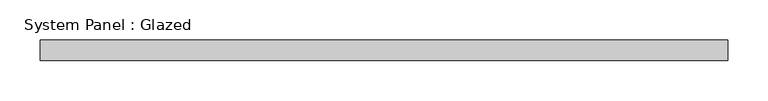
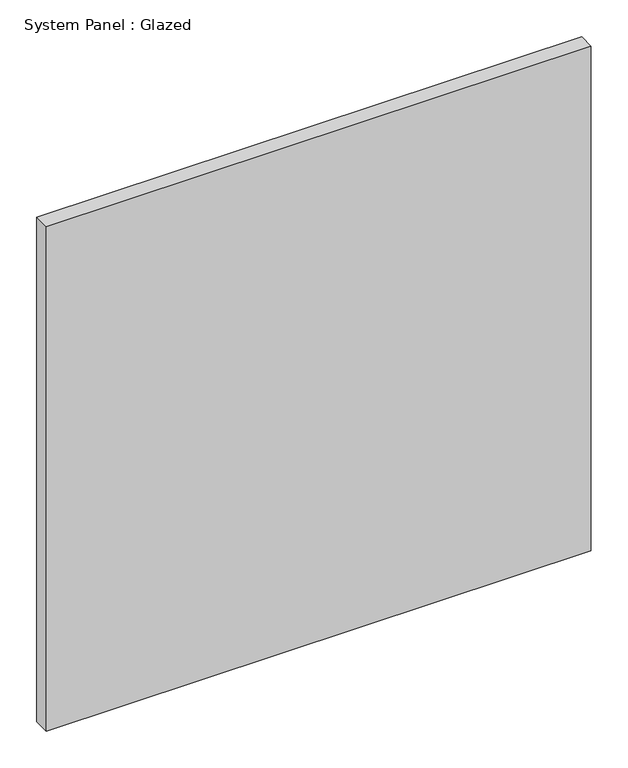
"""IFC4 building model written with IfcOpenShell, lengths in millimetres: plate geometry, System Panel : Glazed."""

from ifc_helpers import new_model, si_unit, origin, origin_with_axes, place, context, project, spatial, polyline, outline, extrude, source, transform, mapped, element, save


def system_panel_glazed_d6f3e944(model_context):
    return source(origin(), model_context, "Body", "SweptSolid", [
        extrude(outline(polyline([(425.45, 19.05), (-425.45, 19.05), (-425.45, 44.45), (425.45, 44.45), (425.45, 19.05)])), origin_with_axes(), (0.0, 0.0, 1.0), 832.1153615),
    ])


if __name__ == "__main__":
    model = new_model("IFC4")
    model_context = context("Model", 3, world=origin())
    ifc_project = project(units=[si_unit("LENGTHUNIT", "METRE", prefix="MILLI")], contexts=[model_context])
    site = spatial("IfcSite", under=ifc_project)
    building = spatial("IfcBuilding", under=site)
    placement = place(None, origin())
    system_panel_glazed_shape = system_panel_glazed_d6f3e944(model_context)
    element("IfcPlate", 1, ObjectType="System Panel : Glazed", at=placement, inside=building, context=model_context, shape_type="MappedRepresentation", body=[
        mapped(system_panel_glazed_shape, transform((0.0, 0.0, 0.0), x_axis=(1.0, 0.0, 0.0), y_axis=(0.0, 1.0, 0.0), z_axis=(0.0, 0.0, 1.0))),
    ])
    save(model, "model.ifc")

# Revit data of these elements
# Type "System Panel : Glazed"
#   Construction Type Id = "GSP4R"
#   Analytic Construction = "1/8 in Pilkington single glazing"
#   Visual Light Transmittance = 0.9
#   Solar Heat Gain Coefficient = 0.86
#   Heat Transfer Coefficient (U) = 1.18115 BTU/(h·ft²·°F)
#   Define Thermal Properties by = 1
# Element 1 (IfcPlate, "System Panel : Glazed")
#   Materials on its faces: "Glass"
# Materials
#   "Glass": class "Glass", colour RGB 0 128 192, transparency 0.75, Description = "Soda Lime Glass", Cost = 0
